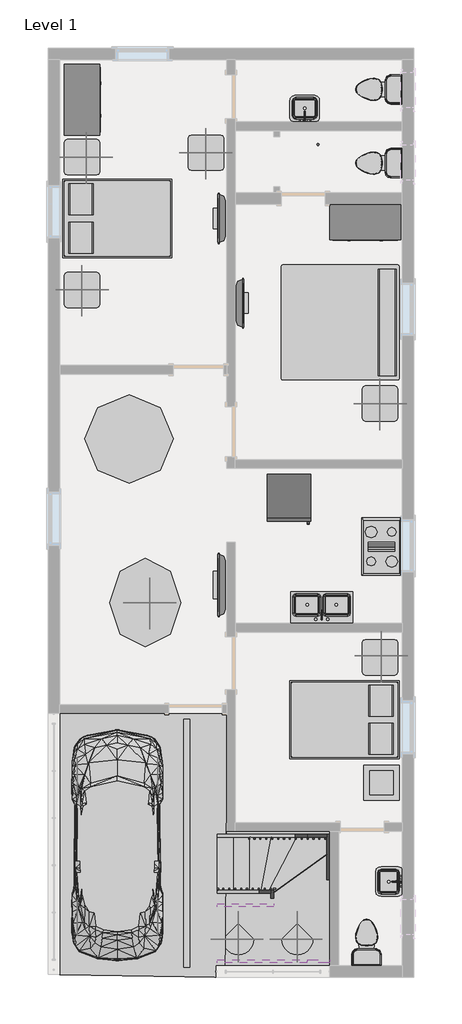
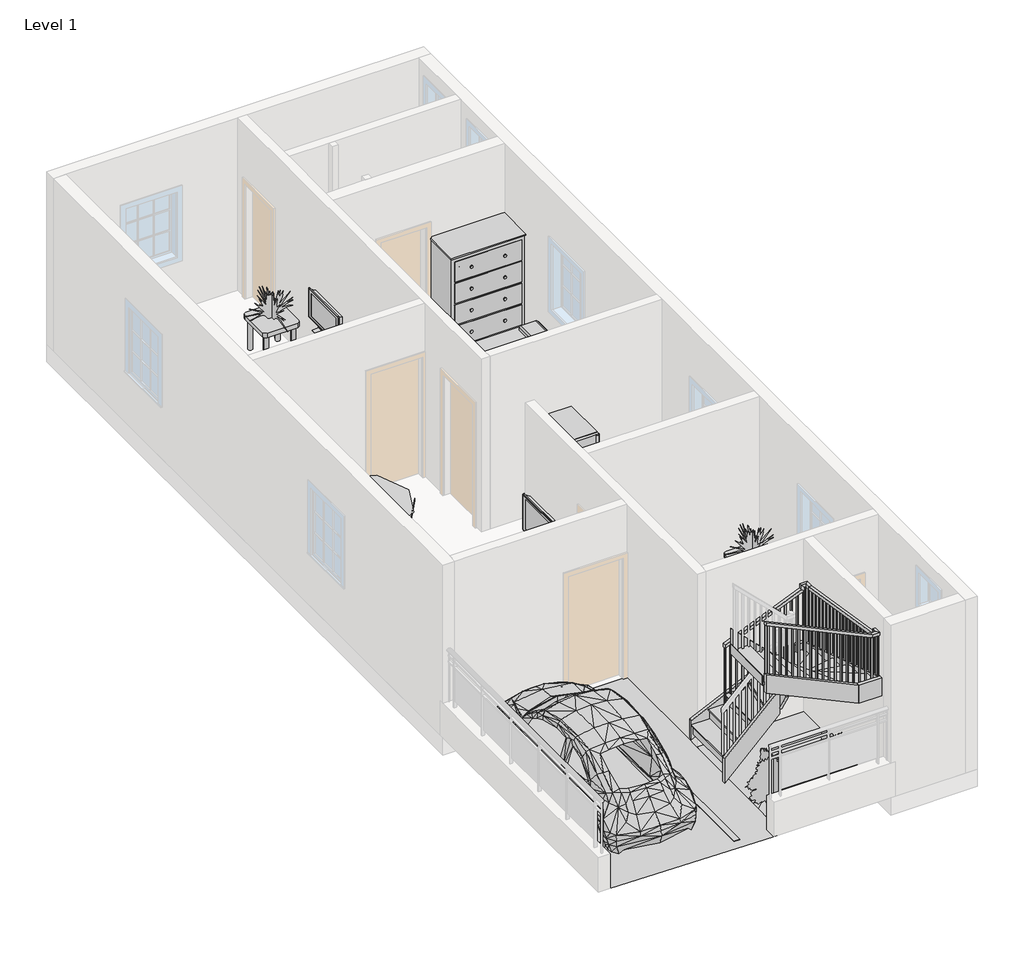
# One storey, part 3 of 3: 16 furniture elements, 10 flow terminals, 8 geographic elements, 8 members, 6 proxies, 1 railing, 1 stair flight.
"""IFC4 building model written with IfcOpenShell, lengths in millimetres."""

from ifc_helpers import new_model, si_unit, frame, origin, place, context, project, spatial, polyline, outline, extrude, faceted_brep, triangles, transform, mapped, element, save
from components import proxy_bb1e6e30, parking_space_9_x_18_90_deg_fdd9e8f5, rpc_beetle_rpc_beetle_3ce7ba48, proxy_a13a33b2, flow_terminal_2b63360b, flow_terminal_accce45a, flow_terminal_a53be723, flow_terminal_d49f872f, flow_terminal_62a433f7, toilet_domestic_3d_toilet_domestic_3d_f7549cf7, toilet_domestic_3d_toilet_domestic_3d_183bbd19, furniture_c8abb964, furniture_1fc5af50, furniture_9fa109b2, furniture_56245f3a, furniture_7a3aaa4f, furniture_b5c51a22, furniture_bbcc68ce, furniture_743965d2, furniture_31d08a24, rpc_plant_tropical_agave_1_5_93a2a214, rpc_plant_tropical_jungle_flame_3_9c4808c2, stair_flight_89efee2b

model = new_model("IFC4")

# Units and contexts
model_context = context("Model", 3, world=origin())
ifc_project = project(units=[si_unit("LENGTHUNIT", "METRE", prefix="MILLI")], contexts=[model_context])

# Site, building, storey
site = spatial("IfcSite", under=ifc_project)
building = spatial("IfcBuilding", under=site)
storey = spatial("IfcBuildingStorey", under=building, Name="Level 1", Elevation=0.0)

# Proxies
placement = place(None, origin())
element("IfcBuildingElementProxy", 1, Name="Building Element Proxy", at=placement, inside=storey, context=model_context, shape_type="Tessellation", body=[
    triangles([(-14717.9109375, 1512.0104702, 0.0), (-11644.5113251, 1512.0104702, 0.0), (-11665.5135315, -2272.5896267, 0.0), (-14514.7117126, -2272.5896267, 0.0), (-14514.7117126, -2983.7896751, 0.0), (-11822.3109375, -3034.5894814, 0.0), (-11675.0896912, -3034.5894814, 0.0)], [[1, 5, 4], [4, 5, 6], [1, 4, 2], [6, 7, 3], [2, 4, 3], [3, 4, 6]], closed=False),
])
element("IfcBuildingElementProxy", 2, Name="Building Element Proxy", at=placement, inside=storey, context=model_context, shape_type="Tessellation", body=[
    triangles([(-11644.5113251, -519.9895904, 0.0), (-9968.1113251, -519.9895904, 0.0), (-9968.1113251, -2272.5896267, 0.0), (-11568.3113251, -2272.5896267, 0.0), (-11664.9972839, -2272.5896267, 0.0), (-11667.5389893, -855.5340437, 0.0), (-9866.5117126, -2475.7895782, 0.0), (-9866.5117126, -519.9895904, 0.0), (-11653.0654541, -2831.3896751, 0.0), (-11670.8166962, -2831.3896751, 0.0), (-9866.5117126, -2831.3896751, 0.0)], [[10, 9, 5], [3, 9, 11], [1, 6, 2], [5, 6, 10], [5, 4, 6], [5, 9, 4], [3, 11, 7], [3, 4, 9], [3, 6, 4], [3, 7, 8], [2, 6, 3], [2, 3, 8]], closed=False),
])
proxy_shape = proxy_bb1e6e30(model_context)
element("IfcBuildingElementProxy", 3, Name="Cook Top-4 Unit : 36\" x 20\"", ObjectType="Cook Top-4 Unit : 36\" x 20\"", at=placement, inside=storey, context=model_context, shape_type="MappedRepresentation", body=[
    mapped(proxy_shape, transform((-8977.5112155, 4382.2104001, 0.0), x_axis=(0.0, -1.0000000000000004, 0.0), y_axis=(1.0000000000000004, 0.0, 0.0), z_axis=(0.0, 0.0, 1.0))),
])
parking_space_9_x_18_90_deg_shape = parking_space_9_x_18_90_deg_fdd9e8f5(model_context)
element("IfcBuildingElementProxy", 4, Name="Parking Space : 9' x 18' - 90 deg", ObjectType="Parking Space : 9' x 18' - 90 deg", at=placement, inside=storey, context=model_context, shape_type="MappedRepresentation", body=[
    mapped(parking_space_9_x_18_90_deg_shape, transform((-12330.3112155, -2856.7895999, 0.0), x_axis=(-1.0000000000000002, 0.0, 0.0), y_axis=(0.0, -1.0000000000000002, 0.0), z_axis=(0.0, 0.0, 1.0))),
])
rpc_beetle_rpc_beetle_shape = rpc_beetle_rpc_beetle_3ce7ba48(model_context)
element("IfcBuildingElementProxy", 5, Name="RPC Beetle : RPC Beetle", ObjectType="RPC Beetle : RPC Beetle", at=placement, inside=storey, context=model_context, shape_type="MappedRepresentation", body=[
    mapped(rpc_beetle_rpc_beetle_shape, transform((-13524.1112155, -1993.1895999, 0.0), x_axis=(1.0, 0.0, 0.0), y_axis=(0.0, 1.0, 0.0), z_axis=(0.0, 0.0, 1.0))),
])
proxy_2_shape = proxy_a13a33b2(model_context)
element("IfcBuildingElementProxy", 6, Name="Refrigerator : 30\" x 32\" RH", ObjectType="Refrigerator : 30\" x 32\" RH", at=placement, inside=storey, context=model_context, shape_type="MappedRepresentation", body=[
    mapped(proxy_2_shape, transform((-10569.7737155, 5238.2614286, 0.0), x_axis=(1.0, 0.0, 0.0), y_axis=(0.0, 1.0, 0.0), z_axis=(0.0, 0.0, 1.0))),
])

# Flow terminals
flow_terminal_shape = flow_terminal_2b63360b(model_context)
element("IfcFlowTerminal", 7, ObjectType="Floor Drain - Rectangular : 5\"x5\" Strainer - 2\" Drain", at=placement, inside=storey, context=model_context, shape_type="MappedRepresentation", body=[
    mapped(flow_terminal_shape, transform((-9587.1112155, 12586.4104001, 0.0), x_axis=(1.0, 0.0, 0.0), y_axis=(0.0, 1.0, 0.0), z_axis=(0.0, 0.0, 1.0))),
])
element("IfcFlowTerminal", 8, ObjectType="Floor Drain - Rectangular : 5\"x5\" Strainer - 2\" Drain", at=placement, inside=storey, context=model_context, shape_type="MappedRepresentation", body=[
    mapped(flow_terminal_shape, transform((-9510.9112155, 11367.2104001, 0.0), x_axis=(1.0, 0.0, 0.0), y_axis=(0.0, 1.0, 0.0), z_axis=(0.0, 0.0, 1.0))),
])
flow_terminal_2_shape = flow_terminal_accce45a(model_context)
element("IfcFlowTerminal", 9, ObjectType="Floor Drain - Round : 5\" Strainer - 2\" Drain", at=placement, inside=storey, context=model_context, shape_type="MappedRepresentation", body=[
    mapped(flow_terminal_2_shape, transform((-8799.7112155, -2145.5895999, 0.0), x_axis=(1.0, 0.0, 0.0), y_axis=(0.0, 1.0, 0.0), z_axis=(0.0, 0.0, 1.0))),
])
flow_terminal_3_shape = flow_terminal_a53be723(model_context)
element("IfcFlowTerminal", 10, ObjectType="Sink Kitchen-Double : 42\" x 21\"", at=placement, inside=storey, context=model_context, shape_type="MappedRepresentation", body=[
    mapped(flow_terminal_3_shape, transform((-9990.521975, 3343.1558012, 0.0), x_axis=(-1.0000000000000004, 0.0, 0.0), y_axis=(0.0, -1.0000000000000004, 0.0), z_axis=(0.0, 0.0, 1.0))),
])
flow_terminal_4_shape = flow_terminal_d49f872f(model_context)
element("IfcFlowTerminal", 11, ObjectType="Sink Vanity-Round : 19\" x 19\"", at=placement, inside=storey, context=model_context, shape_type="MappedRepresentation", body=[
    mapped(flow_terminal_4_shape, transform((-10166.3629561, 11222.9262428, 609.6), x_axis=(1.0000000000000004, 0.0, 0.0), y_axis=(0.0, 1.0000000000000004, 0.0), z_axis=(0.0, 0.0, 1.0))),
])
flow_terminal_5_shape = flow_terminal_62a433f7(model_context)
element("IfcFlowTerminal", 12, ObjectType="Sink Vanity-Square : 20\" x 18\"", at=placement, inside=storey, context=model_context, shape_type="MappedRepresentation", body=[
    mapped(flow_terminal_5_shape, transform((-10282.621975, 11877.5558012, 0.0), x_axis=(-1.0000000000000004, 0.0, 0.0), y_axis=(0.0, -1.0000000000000004, 0.0), z_axis=(0.0, 0.0, 1.0))),
])
element("IfcFlowTerminal", 13, ObjectType="Sink Vanity-Square : 20\" x 18\"", at=placement, inside=storey, context=model_context, shape_type="MappedRepresentation", body=[
    mapped(flow_terminal_5_shape, transform((-8802.0566166, -1367.9003593, 0.0), x_axis=(0.0, -1.0000000000000004, 0.0), y_axis=(1.0000000000000004, 0.0, 0.0), z_axis=(0.0, 0.0, 1.0))),
])
toilet_domestic_3d_toilet_domestic_3d_shape = toilet_domestic_3d_toilet_domestic_3d_f7549cf7(model_context)
toilet_domestic_3d_toilet_domestic_3d_2_shape = toilet_domestic_3d_toilet_domestic_3d_183bbd19(model_context)
element("IfcFlowTerminal", 14, ObjectType="Toilet-Domestic-3D : Toilet-Domestic-3D", at=placement, inside=storey, context=model_context, shape_type="MappedRepresentation", body=[
    mapped(toilet_domestic_3d_toilet_domestic_3d_shape, transform((-9116.6072429, 12256.2104001, 0.0), x_axis=(0.0, -1.0000000000000004, 0.0), y_axis=(1.0000000000000004, 0.0, 0.0), z_axis=(0.0, 0.0, 1.0))),
    mapped(toilet_domestic_3d_toilet_domestic_3d_2_shape, transform((-9116.6072429, 12256.2104001, 0.0), x_axis=(0.0, -1.0000000000000004, 0.0), y_axis=(1.0000000000000004, 0.0, 0.0), z_axis=(0.0, 0.0, 1.0))),
])
element("IfcFlowTerminal", 15, ObjectType="Toilet-Domestic-3D : Toilet-Domestic-3D", at=placement, inside=storey, context=model_context, shape_type="MappedRepresentation", body=[
    mapped(toilet_domestic_3d_toilet_domestic_3d_shape, transform((-9116.6072429, 10986.2104001, 0.0), x_axis=(0.0, -1.0000000000000004, 0.0), y_axis=(1.0000000000000004, 0.0, 0.0), z_axis=(0.0, 0.0, 1.0))),
    mapped(toilet_domestic_3d_toilet_domestic_3d_2_shape, transform((-9116.6072429, 10986.2104001, 0.0), x_axis=(0.0, -1.0000000000000004, 0.0), y_axis=(1.0000000000000004, 0.0, 0.0), z_axis=(0.0, 0.0, 1.0))),
])
element("IfcFlowTerminal", 16, ObjectType="Toilet-Domestic-3D : Toilet-Domestic-3D", at=placement, inside=storey, context=model_context, shape_type="MappedRepresentation", body=[
    mapped(toilet_domestic_3d_toilet_domestic_3d_shape, transform((-9231.5112155, -2336.6935725, 0.0), x_axis=(-1.0000000000000002, 0.0, 0.0), y_axis=(0.0, -1.0000000000000002, 0.0), z_axis=(0.0, 0.0, 1.0))),
    mapped(toilet_domestic_3d_toilet_domestic_3d_2_shape, transform((-9231.5112155, -2336.6935725, 0.0), x_axis=(-1.0000000000000002, 0.0, 0.0), y_axis=(0.0, -1.0000000000000002, 0.0), z_axis=(0.0, 0.0, 1.0))),
])

# Furniture
furniture_shape = furniture_c8abb964(model_context)
element("IfcFurniture", 17, ObjectType="Bed-Box : Double 53\" x 74\"", at=placement, inside=storey, context=model_context, shape_type="MappedRepresentation", body=[
    mapped(furniture_shape, transform((-13758.5407237, 9694.5579411, 0.0), x_axis=(0.0, 1.0000000000000002, 0.0), y_axis=(-1.0000000000000002, 0.0, 0.0), z_axis=(0.0, 0.0, 1.0))),
])
element("IfcFurniture", 18, ObjectType="Bed-Box : Double 53\" x 74\"", at=placement, inside=storey, context=model_context, shape_type="MappedRepresentation", body=[
    mapped(furniture_shape, transform((-9378.0817073, 1740.6104001, 0.0), x_axis=(0.0, -1.0000000000000002, 0.0), y_axis=(1.0000000000000002, 0.0, 0.0), z_axis=(0.0, 0.0, 1.0))),
])
furniture_2_shape = furniture_1fc5af50(model_context)
element("IfcFurniture", 19, ObjectType="Bed-Standard.0001 : King 78\" x 80\"", at=placement, inside=storey, context=model_context, shape_type="MappedRepresentation", body=[
    mapped(furniture_2_shape, transform((-9643.1161336, 8514.4989247, 0.0), x_axis=(0.0, -1.0, 0.0), y_axis=(1.0, 0.0, 0.0), z_axis=(0.0, 0.0, 1.0))),
])
furniture_3_shape = furniture_9fa109b2(model_context)
element("IfcFurniture", 20, ObjectType="Dresser : 48\" x 72\" x 24\"", at=placement, inside=storey, context=model_context, shape_type="MappedRepresentation", body=[
    mapped(furniture_3_shape, transform((-14496.8741696, 12347.6036599, 0.0), x_axis=(0.0, 1.0000000000000002, 0.0), y_axis=(-1.0000000000000002, 0.0, 0.0), z_axis=(0.0, 0.0, 1.0))),
])
element("IfcFurniture", 21, ObjectType="Dresser : 48\" x 72\" x 24\"", at=placement, inside=storey, context=model_context, shape_type="MappedRepresentation", body=[
    mapped(furniture_3_shape, transform((-8987.7179557, 10333.3733542, 0.0), x_axis=(1.0, 0.0, 0.0), y_axis=(0.0, 1.0, 0.0), z_axis=(0.0, 0.0, 1.0))),
])
furniture_4_shape = furniture_56245f3a(model_context)
element("IfcFurniture", 22, ObjectType="TV - Flat Screen : 32\"", at=placement, inside=storey, context=model_context, shape_type="MappedRepresentation", body=[
    mapped(furniture_4_shape, transform((-11722.0998392, 10029.765886, 914.4), x_axis=(0.0, -1.0000000000000002, 0.0), y_axis=(1.0000000000000002, 0.0, 0.0), z_axis=(0.0, 0.0, 1.0))),
])
element("IfcFurniture", 23, ObjectType="TV - Flat Screen : 32\"", at=placement, inside=storey, context=model_context, shape_type="MappedRepresentation", body=[
    mapped(furniture_4_shape, transform((-11420.9593185, 8577.1549142, 914.4), x_axis=(0.0, 1.0000000000000002, 0.0), y_axis=(-1.0000000000000002, 0.0, 0.0), z_axis=(0.0, 0.0, 1.0))),
])
furniture_5_shape = furniture_7a3aaa4f(model_context)
element("IfcFurniture", 24, ObjectType="TV - Flat Screen : 42\"", at=placement, inside=storey, context=model_context, shape_type="MappedRepresentation", body=[
    mapped(furniture_5_shape, transform((-11722.0998392, 3717.865886, 914.4), x_axis=(0.0, -1.0000000000000004, 0.0), y_axis=(1.0000000000000004, 0.0, 0.0), z_axis=(0.0, 0.0, 1.0))),
])
furniture_6_shape = furniture_b5c51a22(model_context)
element("IfcFurniture", 25, ObjectType="Table-Coffee : 24\" x 24\" x 24\"", at=placement, inside=storey, context=model_context, shape_type="MappedRepresentation", body=[
    mapped(furniture_6_shape, transform((-8995.7769822, 222.9993223, 0.0), x_axis=(1.0, 0.0, 0.0), y_axis=(0.0, 1.0, 0.0), z_axis=(0.0, 0.0, 1.0))),
])
furniture_7_shape = furniture_bbcc68ce(model_context)
element("IfcFurniture", 26, ObjectType="Table-Dining Round w Chairs : 60\" Diameter", at=placement, inside=storey, context=model_context, shape_type="MappedRepresentation", body=[
    mapped(furniture_7_shape, transform((-13424.5931827, 6421.2890886, 0.0), x_axis=(1.0, 0.0, 0.0), y_axis=(0.0, 1.0, 0.0), z_axis=(0.0, 0.0, 1.0))),
])
furniture_8_shape = furniture_743965d2(model_context)
element("IfcFurniture", 27, ObjectType="Table-Ellipse : 60\" x 48\"", at=placement, inside=storey, context=model_context, shape_type="MappedRepresentation", body=[
    mapped(furniture_8_shape, transform((-13041.5112155, 3417.0104001, 0.0), x_axis=(0.0, 1.0000000000000002, 0.0), y_axis=(-1.0000000000000002, 0.0, 0.0), z_axis=(0.0, 0.0, 1.0))),
])
furniture_9_shape = furniture_31d08a24(model_context)
element("IfcFurniture", 28, ObjectType="Table-End : 24\" x 24\"", at=placement, inside=storey, context=model_context, shape_type="MappedRepresentation", body=[
    mapped(furniture_9_shape, transform((-14442.2448458, 10935.4104001, 0.0), x_axis=(1.0, 0.0, 0.0), y_axis=(0.0, 1.0, 0.0), z_axis=(0.0, 0.0, 1.0))),
])
element("IfcFurniture", 29, ObjectType="Table-End : 24\" x 24\"", at=placement, inside=storey, context=model_context, shape_type="MappedRepresentation", body=[
    mapped(furniture_9_shape, transform((-14442.2448458, 8649.4104001, 0.0), x_axis=(1.0, 0.0, 0.0), y_axis=(0.0, 1.0, 0.0), z_axis=(0.0, 0.0, 1.0))),
])
element("IfcFurniture", 30, ObjectType="Table-End : 24\" x 24\"", at=placement, inside=storey, context=model_context, shape_type="MappedRepresentation", body=[
    mapped(furniture_9_shape, transform((-12308.6448458, 11011.6104001, 0.0), x_axis=(1.0, 0.0, 0.0), y_axis=(0.0, 1.0, 0.0), z_axis=(0.0, 0.0, 1.0))),
])
element("IfcFurniture", 31, ObjectType="Table-End : 24\" x 24\"", at=placement, inside=storey, context=model_context, shape_type="MappedRepresentation", body=[
    mapped(furniture_9_shape, transform((-9311.4448458, 6693.6104001, 0.0), x_axis=(1.0, 0.0, 0.0), y_axis=(0.0, 1.0, 0.0), z_axis=(0.0, 0.0, 1.0))),
])
element("IfcFurniture", 32, ObjectType="Table-End : 24\" x 24\"", at=placement, inside=storey, context=model_context, shape_type="MappedRepresentation", body=[
    mapped(furniture_9_shape, transform((-9311.4448458, 2324.8104001, 0.0), x_axis=(1.0, 0.0, 0.0), y_axis=(0.0, 1.0, 0.0), z_axis=(0.0, 0.0, 1.0))),
])

# Geographic elements
rpc_plant_tropical_agave_1_5_shape = rpc_plant_tropical_agave_1_5_93a2a214(model_context)
element("IfcGeographicElement", 33, ObjectType="RPC Plant - Tropical : Agave - 1.5'", at=placement, inside=storey, context=model_context, shape_type="MappedRepresentation", body=[
    mapped(rpc_plant_tropical_agave_1_5_shape, transform((-14057.5112155, 11087.8104001, 609.6), x_axis=(1.0, 0.0, 0.0), y_axis=(0.0, 1.0, 0.0), z_axis=(0.0, 0.0, 1.0))),
])
element("IfcGeographicElement", 34, ObjectType="RPC Plant - Tropical : Agave - 1.5'", at=placement, inside=storey, context=model_context, shape_type="MappedRepresentation", body=[
    mapped(rpc_plant_tropical_agave_1_5_shape, transform((-14133.7112155, 8801.8104001, 609.6), x_axis=(1.0, 0.0, 0.0), y_axis=(0.0, 1.0, 0.0), z_axis=(0.0, 0.0, 1.0))),
])
element("IfcGeographicElement", 35, ObjectType="RPC Plant - Tropical : Agave - 1.5'", at=placement, inside=storey, context=model_context, shape_type="MappedRepresentation", body=[
    mapped(rpc_plant_tropical_agave_1_5_shape, transform((-12000.1112155, 11164.0104001, 609.6), x_axis=(1.0, 0.0, 0.0), y_axis=(0.0, 1.0, 0.0), z_axis=(0.0, 0.0, 1.0))),
])
element("IfcGeographicElement", 36, ObjectType="RPC Plant - Tropical : Agave - 1.5'", at=placement, inside=storey, context=model_context, shape_type="MappedRepresentation", body=[
    mapped(rpc_plant_tropical_agave_1_5_shape, transform((-9002.9112155, 6846.0104001, 609.6), x_axis=(1.0, 0.0, 0.0), y_axis=(0.0, 1.0, 0.0), z_axis=(0.0, 0.0, 1.0))),
])
element("IfcGeographicElement", 37, ObjectType="RPC Plant - Tropical : Agave - 1.5'", at=placement, inside=storey, context=model_context, shape_type="MappedRepresentation", body=[
    mapped(rpc_plant_tropical_agave_1_5_shape, transform((-12965.3112155, 3417.0104001, 762.0), x_axis=(1.0, 0.0, 0.0), y_axis=(0.0, 1.0, 0.0), z_axis=(0.0, 0.0, 1.0))),
])
element("IfcGeographicElement", 38, ObjectType="RPC Plant - Tropical : Agave - 1.5'", at=placement, inside=storey, context=model_context, shape_type="MappedRepresentation", body=[
    mapped(rpc_plant_tropical_agave_1_5_shape, transform((-8977.5112155, 2502.6104001, 609.6), x_axis=(1.0, 0.0, 0.0), y_axis=(0.0, 1.0, 0.0), z_axis=(0.0, 0.0, 1.0))),
])
rpc_plant_tropical_jungle_flame_3_shape = rpc_plant_tropical_jungle_flame_3_9c4808c2(model_context)
element("IfcGeographicElement", 39, ObjectType="RPC Plant - Tropical : Jungle Flame - 3'", at=placement, inside=storey, context=model_context, shape_type="MappedRepresentation", body=[
    mapped(rpc_plant_tropical_jungle_flame_3_shape, transform((-11441.3112155, -2374.1895999, 0.0), x_axis=(1.0, 0.0, 0.0), y_axis=(0.0, 1.0, 0.0), z_axis=(0.0, 0.0, 1.0))),
])
element("IfcGeographicElement", 40, ObjectType="RPC Plant - Tropical : Jungle Flame - 3'", at=placement, inside=storey, context=model_context, shape_type="MappedRepresentation", body=[
    mapped(rpc_plant_tropical_jungle_flame_3_shape, transform((-10425.3112155, -2374.1895999, 0.0), x_axis=(1.0, 0.0, 0.0), y_axis=(0.0, 1.0, 0.0), z_axis=(0.0, 0.0, 1.0))),
])

# Members
element("IfcMember", 41, ObjectType="Stringer - 2\" Width", at=placement, inside=storey, context=model_context, shape_type="SweptSolid", body=[
    extrude(outline(polyline([(577.8751786, -11800.6429074), (241.2701641, -11800.6429074), (965.2955504, -10255.5493466), (1301.9005649, -10255.5493466), (577.8751786, -11800.6429074)])), frame((0.0, -621.5895999, 0.0), z_axis=(0.0, 1.0, 0.0), x_axis=(0.0, 0.0, 1.0)), (0.0, 0.0, 1.0), 50.8),
])
element("IfcMember", 42, ObjectType="Stringer - 2\" Width", at=placement, inside=storey, context=model_context, shape_type="SweptSolid", body=[
    extrude(outline(polyline([(-10255.5493466, -621.5895999), (-10255.5493466, -570.7895999), (-9917.3112155, -570.7895999), (-9917.3112155, -621.5895999), (-10255.5493466, -621.5895999)])), frame((0.0, 0.0, 965.2955504), z_axis=(0.0, 0.0, 1.0), x_axis=(1.0, 0.0, 0.0)), (0.0, 0.0, 1.0), 336.6050145),
])
element("IfcMember", 43, ObjectType="Stringer - 2\" Width", at=placement, inside=storey, context=model_context, shape_type="SweptSolid", body=[
    extrude(outline(polyline([(-570.7895999, 1285.6001408), (-570.7895999, 997.1005649), (-720.7093972, 997.1005649), (-2729.7895999, 1641.7631511), (-2729.7895999, 1969.9972697), (-2703.7018424, 1969.9972697), (-570.7895999, 1285.6001408)])), frame((-9917.3112155, 0.0, 0.0), z_axis=(1.0, 0.0, 0.0), x_axis=(0.0, 1.0, 0.0)), (0.0, 0.0, 1.0), 50.8),
])
element("IfcMember", 44, ObjectType="Stringer - 2\" Width", at=placement, inside=storey, context=model_context, shape_type="SweptSolid", body=[
    extrude(outline(polyline([(-9866.5112155, -2729.7895999), (-9866.5112155, -2780.5895999), (-10255.5493466, -2780.5895999), (-10255.5493466, -2729.7895999), (-9866.5112155, -2729.7895999)])), frame((0.0, 0.0, 1649.8904473), z_axis=(0.0, 0.0, 1.0), x_axis=(1.0, 0.0, 0.0)), (0.0, 0.0, 1.0), 320.1068224),
])
element("IfcMember", 45, ObjectType="Stringer - 2\" Width", at=placement, inside=storey, context=model_context, shape_type="SweptSolid", body=[
    extrude(outline(polyline([(1649.8904473, -10255.5493466), (1969.9972697, -10255.5493466), (2694.022656, -11800.6429074), (2373.9158336, -11800.6429074), (1649.8904473, -10255.5493466)])), frame((0.0, -2780.5895999, 0.0), z_axis=(0.0, 1.0, 0.0), x_axis=(0.0, 0.0, 1.0)), (0.0, 0.0, 1.0), 50.8),
])
element("IfcMember", 46, ObjectType="Stringer - 2\" Width", at=placement, inside=storey, context=model_context, shape_type="SweptSolid", body=[
    extrude(outline(polyline([(489.3391875, -11800.6429074), (61.3897561, -11800.6429074), (966.2551233, -10882.5112155), (1394.2045547, -10882.5112155), (489.3391875, -11800.6429074)])), frame((0.0, -1586.7895999, 0.0), z_axis=(0.0, 1.0, 0.0), x_axis=(0.0, 0.0, 1.0)), (0.0, 0.0, 1.0), 50.8),
])
element("IfcMember", 47, ObjectType="Stringer - 2\" Width", at=placement, inside=storey, context=model_context, shape_type="SweptSolid", body=[
    extrude(outline(polyline([(-1535.9895999, 1573.2682978), (-1535.9895999, 1016.3211008), (-1563.063862, 1016.3211008), (-1764.5895999, 1360.465107), (-1764.5895999, 1947.8002622), (-1755.3100853, 1947.8002622), (-1535.9895999, 1573.2682978)])), frame((-10882.5112155, 0.0, 0.0), z_axis=(1.0, 0.0, 0.0), x_axis=(0.0, 1.0, 0.0)), (0.0, 0.0, 1.0), 50.8),
])
element("IfcMember", 48, ObjectType="Stringer - 2\" Width", at=placement, inside=storey, context=model_context, shape_type="SweptSolid", body=[
    extrude(outline(polyline([(1519.8508308, -10831.7112155), (1947.8002622, -10831.7112155), (2902.731607, -11800.6429074), (2474.7821756, -11800.6429074), (1519.8508308, -10831.7112155)])), frame((0.0, -1815.3895999, 0.0), z_axis=(0.0, 1.0, 0.0), x_axis=(0.0, 0.0, 1.0)), (0.0, 0.0, 1.0), 50.8),
])

# Railing
element("IfcRailing", 49, ObjectType="Handrail - Rectangular", at=placement, inside=storey, context=model_context, shape_type="SolidModel", body=[
    faceted_brep([(-11264.9343115, -621.5895999, 1751.3482604), (-11264.9343115, -621.5895999, 1696.2325103), (-11264.9343115, -672.3895999, 1696.2325103), (-11264.9343115, -672.3895999, 1751.3482604), (-9993.5112155, -621.5895999, 2286.4480794), (-9942.7112155, -621.5895999, 2252.7123647), (-9942.7112155, -672.3895999, 2252.7123647), (-9993.5112155, -672.3895999, 2286.4480794), (-9866.5112155, -752.6490579, 2309.5259032), (-9866.5112155, -748.5895999, 2360.3259032), (-9866.5112155, -2602.7895999, 2658.5708374), (-9866.5112155, -2653.5895999, 2615.2889745), (-9917.3112155, -752.6490579, 2309.5259032), (-9917.3112155, -2653.5895999, 2615.2889745), (-9917.3112155, -748.5895999, 2360.3259032), (-9917.3112155, -2602.7895999, 2658.5708374), (-11771.5112155, -2729.7895999, 3571.6748454), (-11771.5112155, -2678.9895999, 3571.6748454), (-11771.5112155, -2678.9895999, 3515.5740097), (-11771.5112155, -2729.7895999, 3515.5740097), (-10004.8233702, -2729.7895999, 2687.7103241), (-9993.5112155, -2729.7895999, 2738.5103241), (-10004.8233702, -2678.9895999, 2687.7103241), (-9993.5112155, -2678.9895999, 2738.5103241), (-9993.5112155, -621.5895999, 2360.3259032), (-9942.7112155, -621.5895999, 2309.5259032), (-9942.7112155, -672.3895999, 2309.5259032), (-9993.5112155, -672.3895999, 2360.3259032), (-9866.5112155, -621.5895999, 2360.3259032), (-9866.5112155, -621.5895999, 2309.5259032), (-9917.3112155, -672.3895999, 2309.5259032), (-9917.3112155, -672.3895999, 2360.3259032), (-9866.5112155, -2602.7895999, 2738.5103241), (-9866.5112155, -2653.5895999, 2687.7103241), (-9917.3112155, -2653.5895999, 2687.7103241), (-9917.3112155, -2602.7895999, 2738.5103241), (-9866.5112155, -2729.7895999, 2738.5103241), (-9866.5112155, -2729.7895999, 2687.7103241), (-9917.3112155, -2678.9895999, 2687.7103241), (-9917.3112155, -2678.9895999, 2738.5103241)], [[[0, 1, 2, 3]], [[1, 0, 4, 5]], [[2, 1, 5, 6]], [[3, 2, 6, 7]], [[0, 3, 7, 4]], [[8, 9, 10, 11]], [[12, 8, 11, 13]], [[14, 12, 13, 15]], [[9, 14, 15, 10]], [[16, 17, 18, 19]], [[20, 21, 16, 19]], [[22, 20, 19, 18]], [[23, 22, 18, 17]], [[21, 23, 17, 16]], [[5, 4, 24, 25]], [[6, 5, 25, 26]], [[7, 6, 26, 27]], [[4, 7, 27, 24]], [[25, 24, 28, 29]], [[26, 25, 29, 30]], [[27, 26, 30, 31]], [[24, 27, 31, 28]], [[29, 28, 9, 8]], [[30, 29, 8, 12]], [[31, 30, 12, 14]], [[28, 31, 14, 9]], [[11, 10, 32, 33]], [[13, 11, 33, 34]], [[15, 13, 34, 35]], [[10, 15, 35, 32]], [[33, 32, 36, 37]], [[34, 33, 37, 38]], [[35, 34, 38, 39]], [[32, 35, 39, 36]], [[37, 36, 21, 20]], [[38, 37, 20, 22]], [[39, 38, 22, 23]], [[36, 39, 23, 21]]]),
    extrude(outline(polyline([(3496.2326904, -11730.2362155), (2540.0, -11730.2362155), (2540.0, -11711.1862155), (3487.3059277, -11711.1862155), (3496.2326904, -11730.2362155)])), frame((0.0, -2713.9145999, 0.0), z_axis=(0.0, 1.0, 0.0), x_axis=(0.0, 0.0, 1.0)), (0.0, 0.0, 1.0), 19.05),
    extrude(outline(polyline([(3448.6232892, -11628.6362155), (2540.0, -11628.6362155), (2540.0, -11609.5862155), (3439.6965265, -11609.5862155), (3448.6232892, -11628.6362155)])), frame((0.0, -2713.9145999, 0.0), z_axis=(0.0, 1.0, 0.0), x_axis=(0.0, 0.0, 1.0)), (0.0, 0.0, 1.0), 19.05),
    extrude(outline(polyline([(3401.013888, -11527.0362155), (2370.6666667, -11527.0362155), (2370.6666667, -11507.9862155), (3392.0871253, -11507.9862155), (3401.013888, -11527.0362155)])), frame((0.0, -2713.9145999, 0.0), z_axis=(0.0, 1.0, 0.0), x_axis=(0.0, 0.0, 1.0)), (0.0, 0.0, 1.0), 19.05),
    extrude(outline(polyline([(3353.4044868, -11425.4362155), (2370.6666667, -11425.4362155), (2370.6666667, -11406.3862155), (3344.477724, -11406.3862155), (3353.4044868, -11425.4362155)])), frame((0.0, -2713.9145999, 0.0), z_axis=(0.0, 1.0, 0.0), x_axis=(0.0, 0.0, 1.0)), (0.0, 0.0, 1.0), 19.05),
    extrude(outline(polyline([(3305.7950856, -11323.8362155), (2370.6666667, -11323.8362155), (2370.6666667, -11304.7862155), (3296.8683228, -11304.7862155), (3305.7950856, -11323.8362155)])), frame((0.0, -2713.9145999, 0.0), z_axis=(0.0, 1.0, 0.0), x_axis=(0.0, 0.0, 1.0)), (0.0, 0.0, 1.0), 19.05),
    extrude(outline(polyline([(3258.1856843, -11222.2362155), (2201.3333333, -11222.2362155), (2201.3333333, -11203.1862155), (3249.2589216, -11203.1862155), (3258.1856843, -11222.2362155)])), frame((0.0, -2713.9145999, 0.0), z_axis=(0.0, 1.0, 0.0), x_axis=(0.0, 0.0, 1.0)), (0.0, 0.0, 1.0), 19.05),
    extrude(outline(polyline([(3210.5762831, -11120.6362155), (2201.3333333, -11120.6362155), (2201.3333333, -11101.5862155), (3201.6495204, -11101.5862155), (3210.5762831, -11120.6362155)])), frame((0.0, -2713.9145999, 0.0), z_axis=(0.0, 1.0, 0.0), x_axis=(0.0, 0.0, 1.0)), (0.0, 0.0, 1.0), 19.05),
    extrude(outline(polyline([(3162.9668819, -11019.0362155), (2201.3333333, -11019.0362155), (2201.3333333, -10999.9862155), (3154.0401192, -10999.9862155), (3162.9668819, -11019.0362155)])), frame((0.0, -2713.9145999, 0.0), z_axis=(0.0, 1.0, 0.0), x_axis=(0.0, 0.0, 1.0)), (0.0, 0.0, 1.0), 19.05),
    extrude(outline(polyline([(3115.3574807, -10917.4362155), (2201.3333333, -10917.4362155), (2201.3333333, -10898.3862155), (3106.430718, -10898.3862155), (3115.3574807, -10917.4362155)])), frame((0.0, -2713.9145999, 0.0), z_axis=(0.0, 1.0, 0.0), x_axis=(0.0, 0.0, 1.0)), (0.0, 0.0, 1.0), 19.05),
    extrude(outline(polyline([(3067.7480795, -10815.8362155), (2032.0, -10815.8362155), (2032.0, -10796.7862155), (3058.8213168, -10796.7862155), (3067.7480795, -10815.8362155)])), frame((0.0, -2713.9145999, 0.0), z_axis=(0.0, 1.0, 0.0), x_axis=(0.0, 0.0, 1.0)), (0.0, 0.0, 1.0), 19.05),
    extrude(outline(polyline([(3020.1386783, -10714.2362155), (2032.0, -10714.2362155), (2032.0, -10695.1862155), (3011.2119155, -10695.1862155), (3020.1386783, -10714.2362155)])), frame((0.0, -2713.9145999, 0.0), z_axis=(0.0, 1.0, 0.0), x_axis=(0.0, 0.0, 1.0)), (0.0, 0.0, 1.0), 19.05),
    extrude(outline(polyline([(2972.5292771, -10612.6362155), (2032.0, -10612.6362155), (2032.0, -10593.5862155), (2963.6025143, -10593.5862155), (2972.5292771, -10612.6362155)])), frame((0.0, -2713.9145999, 0.0), z_axis=(0.0, 1.0, 0.0), x_axis=(0.0, 0.0, 1.0)), (0.0, 0.0, 1.0), 19.05),
    extrude(outline(polyline([(2924.9198758, -10511.0362155), (2032.0, -10511.0362155), (2032.0, -10491.9862155), (2915.9931131, -10491.9862155), (2924.9198758, -10511.0362155)])), frame((0.0, -2713.9145999, 0.0), z_axis=(0.0, 1.0, 0.0), x_axis=(0.0, 0.0, 1.0)), (0.0, 0.0, 1.0), 19.05),
    extrude(outline(polyline([(2877.3104746, -10409.4362155), (1862.6666667, -10409.4362155), (1862.6666667, -10390.3862155), (2868.3837119, -10390.3862155), (2877.3104746, -10409.4362155)])), frame((0.0, -2713.9145999, 0.0), z_axis=(0.0, 1.0, 0.0), x_axis=(0.0, 0.0, 1.0)), (0.0, 0.0, 1.0), 19.05),
    extrude(outline(polyline([(2829.7010734, -10307.8362155), (1862.6666667, -10307.8362155), (1862.6666667, -10288.7862155), (2820.7743107, -10288.7862155), (2829.7010734, -10307.8362155)])), frame((0.0, -2713.9145999, 0.0), z_axis=(0.0, 1.0, 0.0), x_axis=(0.0, 0.0, 1.0)), (0.0, 0.0, 1.0), 19.05),
    extrude(outline(polyline([(2782.0916722, -10206.2362155), (1862.6666667, -10206.2362155), (1862.6666667, -10187.1862155), (2773.1649095, -10187.1862155), (2782.0916722, -10206.2362155)])), frame((0.0, -2713.9145999, 0.0), z_axis=(0.0, 1.0, 0.0), x_axis=(0.0, 0.0, 1.0)), (0.0, 0.0, 1.0), 19.05),
    extrude(outline(polyline([(2734.482271, -10104.6362155), (1862.6666667, -10104.6362155), (1862.6666667, -10085.5862155), (2725.5555082, -10085.5862155), (2734.482271, -10104.6362155)])), frame((0.0, -2713.9145999, 0.0), z_axis=(0.0, 1.0, 0.0), x_axis=(0.0, 0.0, 1.0)), (0.0, 0.0, 1.0), 19.05),
    extrude(outline(polyline([(-9983.9862155, -2713.9145999), (-10003.0362155, -2713.9145999), (-10003.0362155, -2694.8645999), (-9983.9862155, -2694.8645999), (-9983.9862155, -2713.9145999)])), frame((0.0, 0.0, 1862.6666667), z_axis=(0.0, 0.0, 1.0), x_axis=(1.0, 0.0, 0.0)), (0.0, 0.0, 1.0), 825.0436575),
    extrude(outline(polyline([(-2669.4645999, 2687.7103241), (-2669.4645999, 1959.011412), (-2688.5145999, 1965.124071), (-2688.5145999, 2687.7103241), (-2669.4645999, 2687.7103241)])), frame((-9901.4362155, 0.0, 0.0), z_axis=(1.0, 0.0, 0.0), x_axis=(0.0, 1.0, 0.0)), (0.0, 0.0, 1.0), 19.05),
    extrude(outline(polyline([(-2567.8645999, 2601.5002533), (-2567.8645999, 1926.4105637), (-2586.9145999, 1932.5232228), (-2586.9145999, 2604.5644135), (-2567.8645999, 2601.5002533)])), frame((-9901.4362155, 0.0, 0.0), z_axis=(1.0, 0.0, 0.0), x_axis=(0.0, 1.0, 0.0)), (0.0, 0.0, 1.0), 19.05),
    extrude(outline(polyline([(-2466.2645999, 2585.1580651), (-2466.2645999, 1893.8097155), (-2485.3145999, 1899.9223745), (-2485.3145999, 2588.2222254), (-2466.2645999, 2585.1580651)])), frame((-9901.4362155, 0.0, 0.0), z_axis=(1.0, 0.0, 0.0), x_axis=(0.0, 1.0, 0.0)), (0.0, 0.0, 1.0), 19.05),
    extrude(outline(polyline([(-2364.6645999, 2568.8158769), (-2364.6645999, 1861.2088673), (-2383.7145999, 1867.3215263), (-2383.7145999, 2571.8800372), (-2364.6645999, 2568.8158769)])), frame((-9901.4362155, 0.0, 0.0), z_axis=(1.0, 0.0, 0.0), x_axis=(0.0, 1.0, 0.0)), (0.0, 0.0, 1.0), 19.05),
    extrude(outline(polyline([(-2263.0645999, 2552.4736887), (-2263.0645999, 1828.608019), (-2282.1145999, 1834.7206781), (-2282.1145999, 2555.537849), (-2263.0645999, 2552.4736887)])), frame((-9901.4362155, 0.0, 0.0), z_axis=(1.0, 0.0, 0.0), x_axis=(0.0, 1.0, 0.0)), (0.0, 0.0, 1.0), 19.05),
    extrude(outline(polyline([(-2161.4645999, 2536.1315006), (-2161.4645999, 1796.0071708), (-2180.5145999, 1802.1198299), (-2180.5145999, 2539.1956608), (-2161.4645999, 2536.1315006)])), frame((-9901.4362155, 0.0, 0.0), z_axis=(1.0, 0.0, 0.0), x_axis=(0.0, 1.0, 0.0)), (0.0, 0.0, 1.0), 19.05),
    extrude(outline(polyline([(-2059.8645999, 2519.7893124), (-2059.8645999, 1763.4063226), (-2078.9145999, 1769.5189816), (-2078.9145999, 2522.8534727), (-2059.8645999, 2519.7893124)])), frame((-9901.4362155, 0.0, 0.0), z_axis=(1.0, 0.0, 0.0), x_axis=(0.0, 1.0, 0.0)), (0.0, 0.0, 1.0), 19.05),
    extrude(outline(polyline([(-1958.2645999, 2503.4471242), (-1958.2645999, 1730.8054744), (-1977.3145999, 1736.9181334), (-1977.3145999, 2506.5112845), (-1958.2645999, 2503.4471242)])), frame((-9901.4362155, 0.0, 0.0), z_axis=(1.0, 0.0, 0.0), x_axis=(0.0, 1.0, 0.0)), (0.0, 0.0, 1.0), 19.05),
    extrude(outline(polyline([(-1856.6645999, 2487.104936), (-1856.6645999, 1698.2046261), (-1875.7145999, 1704.3172852), (-1875.7145999, 2490.1690963), (-1856.6645999, 2487.104936)])), frame((-9901.4362155, 0.0, 0.0), z_axis=(1.0, 0.0, 0.0), x_axis=(0.0, 1.0, 0.0)), (0.0, 0.0, 1.0), 19.05),
    extrude(outline(polyline([(-1755.0645999, 2470.7627479), (-1755.0645999, 1665.6037779), (-1774.1145999, 1671.716437), (-1774.1145999, 2473.8269081), (-1755.0645999, 2470.7627479)])), frame((-9901.4362155, 0.0, 0.0), z_axis=(1.0, 0.0, 0.0), x_axis=(0.0, 1.0, 0.0)), (0.0, 0.0, 1.0), 19.05),
    extrude(outline(polyline([(-1653.4645999, 2454.4205597), (-1653.4645999, 1633.0029297), (-1672.5145999, 1639.1155887), (-1672.5145999, 2457.48472), (-1653.4645999, 2454.4205597)])), frame((-9901.4362155, 0.0, 0.0), z_axis=(1.0, 0.0, 0.0), x_axis=(0.0, 1.0, 0.0)), (0.0, 0.0, 1.0), 19.05),
    extrude(outline(polyline([(-1551.8645999, 2438.0783715), (-1551.8645999, 1600.4020815), (-1570.9145999, 1606.5147405), (-1570.9145999, 2441.1425318), (-1551.8645999, 2438.0783715)])), frame((-9901.4362155, 0.0, 0.0), z_axis=(1.0, 0.0, 0.0), x_axis=(0.0, 1.0, 0.0)), (0.0, 0.0, 1.0), 19.05),
    extrude(outline(polyline([(-1450.2645999, 2421.7361833), (-1450.2645999, 1567.8012332), (-1469.3145999, 1573.9138923), (-1469.3145999, 2424.8003436), (-1450.2645999, 2421.7361833)])), frame((-9901.4362155, 0.0, 0.0), z_axis=(1.0, 0.0, 0.0), x_axis=(0.0, 1.0, 0.0)), (0.0, 0.0, 1.0), 19.05),
    extrude(outline(polyline([(-1348.6645999, 2405.3939951), (-1348.6645999, 1535.200385), (-1367.7145999, 1541.313044), (-1367.7145999, 2408.4581554), (-1348.6645999, 2405.3939951)])), frame((-9901.4362155, 0.0, 0.0), z_axis=(1.0, 0.0, 0.0), x_axis=(0.0, 1.0, 0.0)), (0.0, 0.0, 1.0), 19.05),
    extrude(outline(polyline([(-1247.0645999, 2389.051807), (-1247.0645999, 1502.5995368), (-1266.1145999, 1508.7121958), (-1266.1145999, 2392.1159673), (-1247.0645999, 2389.051807)])), frame((-9901.4362155, 0.0, 0.0), z_axis=(1.0, 0.0, 0.0), x_axis=(0.0, 1.0, 0.0)), (0.0, 0.0, 1.0), 19.05),
    extrude(outline(polyline([(-1145.4645999, 2372.7096188), (-1145.4645999, 1469.9986885), (-1164.5145999, 1476.1113476), (-1164.5145999, 2375.7737791), (-1145.4645999, 2372.7096188)])), frame((-9901.4362155, 0.0, 0.0), z_axis=(1.0, 0.0, 0.0), x_axis=(0.0, 1.0, 0.0)), (0.0, 0.0, 1.0), 19.05),
    extrude(outline(polyline([(-1043.8645999, 2356.3674306), (-1043.8645999, 1437.3978403), (-1062.9145999, 1443.5104994), (-1062.9145999, 2359.4315909), (-1043.8645999, 2356.3674306)])), frame((-9901.4362155, 0.0, 0.0), z_axis=(1.0, 0.0, 0.0), x_axis=(0.0, 1.0, 0.0)), (0.0, 0.0, 1.0), 19.05),
    extrude(outline(polyline([(-942.2645999, 2340.0252424), (-942.2645999, 1404.7969921), (-961.3145999, 1410.9096511), (-961.3145999, 2343.0894027), (-942.2645999, 2340.0252424)])), frame((-9901.4362155, 0.0, 0.0), z_axis=(1.0, 0.0, 0.0), x_axis=(0.0, 1.0, 0.0)), (0.0, 0.0, 1.0), 19.05),
    extrude(outline(polyline([(-840.6645999, 2323.6830543), (-840.6645999, 1372.1961439), (-859.7145999, 1378.3088029), (-859.7145999, 2326.7472145), (-840.6645999, 2323.6830543)])), frame((-9901.4362155, 0.0, 0.0), z_axis=(1.0, 0.0, 0.0), x_axis=(0.0, 1.0, 0.0)), (0.0, 0.0, 1.0), 19.05),
    extrude(outline(polyline([(-739.0645999, 2309.5259032), (-739.0645999, 1339.5952956), (-758.1145999, 1345.7079547), (-758.1145999, 2309.5259032), (-739.0645999, 2309.5259032)])), frame((-9901.4362155, 0.0, 0.0), z_axis=(1.0, 0.0, 0.0), x_axis=(0.0, 1.0, 0.0)), (0.0, 0.0, 1.0), 19.05),
    extrude(outline(polyline([(2248.1046741, -9953.6593115), (1185.3333333, -9953.6593115), (1185.3333333, -9934.6093115), (2256.1221874, -9934.6093115), (2248.1046741, -9953.6593115)])), frame((0.0, -656.5145999, 0.0), z_axis=(0.0, 1.0, 0.0), x_axis=(0.0, 0.0, 1.0)), (0.0, 0.0, 1.0), 19.05),
    extrude(outline(polyline([(2205.3446033, -10055.2593115), (1185.3333333, -10055.2593115), (1185.3333333, -10036.2093115), (2213.3621166, -10036.2093115), (2205.3446033, -10055.2593115)])), frame((0.0, -656.5145999, 0.0), z_axis=(0.0, 1.0, 0.0), x_axis=(0.0, 0.0, 1.0)), (0.0, 0.0, 1.0), 19.05),
    extrude(outline(polyline([(2162.5845325, -10156.8593115), (1185.3333333, -10156.8593115), (1185.3333333, -10137.8093115), (2170.6020458, -10137.8093115), (2162.5845325, -10156.8593115)])), frame((0.0, -656.5145999, 0.0), z_axis=(0.0, 1.0, 0.0), x_axis=(0.0, 0.0, 1.0)), (0.0, 0.0, 1.0), 19.05),
    extrude(outline(polyline([(2119.8244617, -10258.4593115), (1185.3333333, -10258.4593115), (1185.3333333, -10239.4093115), (2127.841975, -10239.4093115), (2119.8244617, -10258.4593115)])), frame((0.0, -656.5145999, 0.0), z_axis=(0.0, 1.0, 0.0), x_axis=(0.0, 0.0, 1.0)), (0.0, 0.0, 1.0), 19.05),
    extrude(outline(polyline([(2077.0643909, -10360.0593115), (1185.3333333, -10360.0593115), (1185.3333333, -10341.0093115), (2085.0819042, -10341.0093115), (2077.0643909, -10360.0593115)])), frame((0.0, -656.5145999, 0.0), z_axis=(0.0, 1.0, 0.0), x_axis=(0.0, 0.0, 1.0)), (0.0, 0.0, 1.0), 19.05),
    extrude(outline(polyline([(2034.3043201, -10461.6593115), (1016.0, -10461.6593115), (1016.0, -10442.6093115), (2042.3218334, -10442.6093115), (2034.3043201, -10461.6593115)])), frame((0.0, -656.5145999, 0.0), z_axis=(0.0, 1.0, 0.0), x_axis=(0.0, 0.0, 1.0)), (0.0, 0.0, 1.0), 19.05),
    extrude(outline(polyline([(1991.5442493, -10563.2593115), (1016.0, -10563.2593115), (1016.0, -10544.2093115), (1999.5617626, -10544.2093115), (1991.5442493, -10563.2593115)])), frame((0.0, -656.5145999, 0.0), z_axis=(0.0, 1.0, 0.0), x_axis=(0.0, 0.0, 1.0)), (0.0, 0.0, 1.0), 19.05),
    extrude(outline(polyline([(1948.7841785, -10664.8593115), (1016.0, -10664.8593115), (1016.0, -10645.8093115), (1956.8016918, -10645.8093115), (1948.7841785, -10664.8593115)])), frame((0.0, -656.5145999, 0.0), z_axis=(0.0, 1.0, 0.0), x_axis=(0.0, 0.0, 1.0)), (0.0, 0.0, 1.0), 19.05),
    extrude(outline(polyline([(1906.0241077, -10766.4593115), (1016.0, -10766.4593115), (1016.0, -10747.4093115), (1914.0416209, -10747.4093115), (1906.0241077, -10766.4593115)])), frame((0.0, -656.5145999, 0.0), z_axis=(0.0, 1.0, 0.0), x_axis=(0.0, 0.0, 1.0)), (0.0, 0.0, 1.0), 19.05),
    extrude(outline(polyline([(1863.2640369, -10868.0593115), (1016.0, -10868.0593115), (1016.0, -10849.0093115), (1871.2815501, -10849.0093115), (1863.2640369, -10868.0593115)])), frame((0.0, -656.5145999, 0.0), z_axis=(0.0, 1.0, 0.0), x_axis=(0.0, 0.0, 1.0)), (0.0, 0.0, 1.0), 19.05),
    extrude(outline(polyline([(1820.503966, -10969.6593115), (846.6666667, -10969.6593115), (846.6666667, -10950.6093115), (1828.5214793, -10950.6093115), (1820.503966, -10969.6593115)])), frame((0.0, -656.5145999, 0.0), z_axis=(0.0, 1.0, 0.0), x_axis=(0.0, 0.0, 1.0)), (0.0, 0.0, 1.0), 19.05),
    extrude(outline(polyline([(1777.7438952, -11071.2593115), (846.6666667, -11071.2593115), (846.6666667, -11052.2093115), (1785.7614085, -11052.2093115), (1777.7438952, -11071.2593115)])), frame((0.0, -656.5145999, 0.0), z_axis=(0.0, 1.0, 0.0), x_axis=(0.0, 0.0, 1.0)), (0.0, 0.0, 1.0), 19.05),
    extrude(outline(polyline([(1734.9838244, -11172.8593115), (846.6666667, -11172.8593115), (846.6666667, -11153.8093115), (1743.0013377, -11153.8093115), (1734.9838244, -11172.8593115)])), frame((0.0, -656.5145999, 0.0), z_axis=(0.0, 1.0, 0.0), x_axis=(0.0, 0.0, 1.0)), (0.0, 0.0, 1.0), 19.05),
    extrude(outline(polyline([(-9882.3862155, -2713.9145999), (-9901.4362155, -2713.9145999), (-9901.4362155, -2694.8645999), (-9882.3862155, -2694.8645999), (-9882.3862155, -2713.9145999)])), frame((0.0, 0.0, 1969.9972697), z_axis=(0.0, 0.0, 1.0), x_axis=(1.0, 0.0, 0.0)), (0.0, 0.0, 1.0), 717.7130545),
    extrude(outline(polyline([(-637.4645999, 2309.5259032), (-637.4645999, 1306.9944474), (-656.5145999, 1313.1071065), (-656.5145999, 2309.5259032), (-637.4645999, 2309.5259032)])), frame((-9901.4362155, 0.0, 0.0), z_axis=(1.0, 0.0, 0.0), x_axis=(0.0, 1.0, 0.0)), (0.0, 0.0, 1.0), 19.05),
    extrude(outline(polyline([(3515.5740097, -11771.5112155), (2540.0, -11771.5112155), (2540.0, -11752.4612155), (3506.6472469, -11752.4612155), (3515.5740097, -11771.5112155)])), frame((0.0, -2713.9145999, 0.0), z_axis=(0.0, 1.0, 0.0), x_axis=(0.0, 0.0, 1.0)), (0.0, 0.0, 1.0), 19.05),
    extrude(outline(polyline([(1696.2325103, -11264.9343115), (677.3333333, -11264.9343115), (677.3333333, -11245.8843115), (1704.2500235, -11245.8843115), (1696.2325103, -11264.9343115)])), frame((0.0, -656.5145999, 0.0), z_axis=(0.0, 1.0, 0.0), x_axis=(0.0, 0.0, 1.0)), (0.0, 0.0, 1.0), 19.05),
])

# Stair flight
stair_flight_shape = stair_flight_89efee2b(model_context)
element("IfcStairFlight", 50, ObjectType="2\" Tread 1\" Nosing 1/4\" Riser", at=placement, inside=storey, context=model_context, shape_type="MappedRepresentation", body=[
    mapped(stair_flight_shape, transform((0.0, 0.0, 0.0), x_axis=(1.0, 0.0, 0.0), y_axis=(0.0, 1.0, 0.0), z_axis=(0.0, 0.0, 1.0))),
])

save(model, "model.ifc")

# Revit data of these elements
# Type "Cook Top-4 Unit : 36\" x 20\""
#   Assembly Code = "E1090400"
#   Depth = 2' - 0"
#   Width = 3' - 0"
#   Burner Material = Steel, Chrome Plated
#   Cooktop Material = Steel, Polished
#   Default Elevation = 0
# Type "Parking Space : 9' x 18' - 90 deg"
#   Angle = 90.00°
#   Parking Length = 18' - 0"
#   Parking Width = 9' - 0"
#   pl = 14' - 0"
#   pw = 7' - 0"
# Type "RPC Beetle : RPC Beetle"
#   built-in parameter 1005195 = "RPC-16-0U6E-L4EG-ENH1-J3KF-SVEL-0TX4-C0"
#   Height = 0
# Type "Refrigerator : 30\" x 32\" RH"
#   Label = "REF."
#   Assembly Code = "E1090400"
#   Depth = 2' - 7 3/4"
#   Handle = 2' - 3"
#   Height = 5' - 10"
#   Rear Clearance = 0' - 2"
#   Top Door Height = 1' - 8"
#   Width = 2' - 5 3/8"
#   Material = Steel, Paint Finish, Ivory, Glossy
#   Default Elevation = 0
# Type "Floor Drain - Rectangular : 5\"x5\" Strainer - 2\" Drain"
#   WFU = 2
#   Strainer Height = 0' - 3 1/4"
#   Half Strainer Length = 0' - 2 1/2"
#   Strainer Length = 0' - 5"
#   Radius 2 = 0' - 3.04167"
#   Radius 1 = 0' - 2.02083"
#   Radius 3 = 0' - 2 1/32"
#   Pipe Radius = 1"
#   Pipe Diameter = 2"
#   Height 2 = 0' - 0.725"
#   Height 1 = 0' - 1 13/16"
#   Body Radius = 0' - 4 1/16"
#   Body Height = 0' - 3 5/8"
#   Body Diameter = 0' - 8 1/8"
#   Drain Material = none
#   HWFU = 0
#   Default Elevation = 0
#   CWFU = 0
# Type "Floor Drain - Round : 5\" Strainer - 2\" Drain"
#   WFU = 2
#   Strainer Height = 0' - 3 1/4"
#   Strainer Radius = 0' - 2 1/2"
#   Strainer Diameter = 0' - 5"
#   Radius 6 = 0' - 0 5/8"
#   Radius 5 = 0' - 1 1/4"
#   Radius 4 = 0' - 1 7/8"
#   Radius 2 = 0' - 3.04167"
#   Radius 1 = 0' - 2.02083"
#   Radius 3 = 0' - 2 1/32"
#   Pipe Radius = 1"
#   Pipe Diameter = 2"
#   Height 2 = 0' - 0.725"
#   Height 1 = 0' - 1 13/16"
#   Body Radius = 0' - 4 1/16"
#   Body Height = 0' - 3 5/8"
#   Body Diameter = 0' - 8 1/8"
#   Drain Material = none
#   HWFU = 0
#   Default Elevation = 0
#   CWFU = 0
# Type "Sink Kitchen-Double : 42\" x 21\""
#   Assembly Code = "D2010410"
#   Counter Height = 3' - 0"
#   Depth = 1' - 9"
#   Width = 3' - 6"
#   Faucet Material = Steel, Polished
#   Sink Material = Steel, Polished
#   Default Elevation = 0
# Type "Sink Vanity-Round : 19\" x 19\""
#   Assembly Code = "D2010400"
#   Top Of Counter = 2' - 7"
#   Basin Material = Porcelain, Linen
#   Faucet Material = Steel, Polished
#   Default Elevation = 0
# Type "Sink Vanity-Square : 20\" x 18\""
#   Assembly Code = "D2010400"
#   Counter Height = 2' - 7"
#   Depth = 1' - 6"
#   Width = 1' - 8"
#   Basin Material = Porcelain, Linen
#   Faucet Material = Steel, Polished
#   Default Elevation = 0
# Type "Toilet-Domestic-3D : Toilet-Domestic-3D"
#   Assembly Code = "D2010110"
#   Toilet - Bowl/Basin Material = Porcelain, Linen
#   Toilet - Seat Material = Laminate, Linen, Matte
#   Default Elevation = 0
# Type "Bed-Box : Double 53\" x 74\""
#   Assembly Code = "E2020200"
#   Length = 6' - 2"
#   Width = 4' - 5"
#   Frame Material = Birch
#   Mattress Material = Linen, White
#   Default Elevation = 0
# Type "Bed-Standard.0001 : King 78\" x 80\""
#   Assembly Code = "E2020200"
#   Length = 6' - 8"
#   Width = 6' - 6"
#   Leg Material = Steel, Chrome Plated
#   Mattress Material = Linen, White
#   Default Elevation = 0
# Type "Dresser : 48\" x 72\" x 24\""
#   Assembly Code = "E2020200"
#   Depth = 2' - 0"
#   Height = 6' - 0"
#   Width = 4' - 0"
#   Dresser Material = Laminate - Ivory, Glossy
#   Drawer Material = Laminate, Ivory, Matte
#   Knob Material = Cherry
#   Default Elevation = 0
# Type "TV - Flat Screen : 32\""
#   SinAng = 0' - 0.0193"
#   L = 2' - 3.79372"
#   H = 1' - 3.6354"
#   Thickness = 0' - 4.33071"
#   Diagonal = 2' - 7.88976"
#   CosAng = 0' - 0.03431"
#   Stand [instance default] = yes
#   Default Elevation = 0
# Type "TV - Flat Screen : 42\""
#   SinAng = 0' - 0.0193"
#   L = 3' - 0.71517"
#   H = 1' - 8.65418"
#   Thickness = 0' - 4.33071"
#   Diagonal = 3' - 6.12598"
#   CosAng = 0' - 0.03431"
#   Stand [instance default] = yes
#   Default Elevation = 0
# Type "Table-Coffee : 24\" x 24\" x 24\""
#   Assembly Code = "E2020200"
#   Height = 2' - 0"
#   Length = 2' - 0"
#   Width = 2' - 0"
#   Top Material = none
#   Frame Material = none
#   Default Elevation = 0
# Type "Table-Dining Round w Chairs : 60\" Diameter"
#   Assembly Code = "E2020200"
#   Radius = 2' - 6"
#   Diameter = 5' - 0"
#   Height = 2' - 6"
#   Chairs = 6
#   Base Material = Pine
#   Top Material = Laminate, Linen, Matte
#   Default Elevation = 0
# Type "Table-Ellipse : 60\" x 48\""
#   Assembly Code = "E2020200"
#   Half Width = 2' - 0"
#   Half Length = 2' - 6"
#   Height = 2' - 6"
#   Length = 5' - 0"
#   Width = 4' - 0"
#   Base Material = Birch
#   Top Material = Birch
#   Default Elevation = 0
# Type "Table-End : 24\" x 24\""
#   Assembly Code = "E2020200"
#   Height = 2' - 0"
#   Length = 2' - 0"
#   Width = 2' - 0"
#   Base Material = Birch
#   Top Material = Laminate, Ivory, Matte
#   Default Elevation = 0
# Type "RPC Plant - Tropical : Agave - 1.5'"
#   built-in parameter 1005198 = "{2, 15},{39, RPC-16-G1GJ-63FX-7K5P-N000-ST1L-LVER-AU},{1, 0},{1, 0},{2, 13},{1, 8},{5, Color},{1, 0},{1, 0},{3, 0.8},{3, 0.8},{3, 0.8},{1, 8},{7, BBoxMin},{1, 0},{1, 0},{1, 0},{1, 0},{1, 0},{1, 8},{7, BBoxMax},{1, 0},{1, 0},{1, 0},{1, 0},{1, 0},{2, 11},{9, RPCTypeId},{1, 0},{1, 0},{39, RPC-16-G1GJ-63FX-7K5P-N000-ST1L-LVER-AU},{1, 6},{14, RPCPlantHeight},{1, 0},{1, 0},{3, 1.5},{2, 11},{7, keyword},{1, 0},{1, 0},{35, :RPCs:Plants [General]:Geometry:RPC},{2, 11},{8, category},{1, 0},{1, 0},{16, Plants [General]},{2, 11},{12, LocalizedUID},{1, 0},{1, 0},{5, Agave},{2, 14},{6, Height},{1, 0},{1, 0},{3, 1.5},{1, 2},{16, Cast Reflections},{1, 0},{1, 0},{1, 0},{1, 2},{12, Cast Shadows},{1, 0},{1, 0},{1, 1},{1, 2},{9, Lock View},{1, 0},{1, 0},{1, 0},{1, 4},{5, ViewC},{1, 0},{1, 0},{1, 0},{21, assetlibrary_base.fbx},{1, 5},"
#   built-in parameter 1005195 = "RPC-16-G1GJ-63FX-7K5P-N000-ST1L-LVER-AU"
#   Type Comments = "Agave"
#   Assembly Code = "G2050500"
#   Height = 1' - 6"
#   Default Elevation = 0
# Type "RPC Plant - Tropical : Jungle Flame - 3'"
#   built-in parameter 1005198 = "{2, 15},{39, RPC-16-FUVJ-JWG0-MWGK-8000-ST1L-LVER-AU},{1, 0},{1, 0},{2, 13},{1, 8},{5, Color},{1, 0},{1, 0},{3, 0.8},{3, 0.8},{3, 0.8},{1, 8},{7, BBoxMin},{1, 0},{1, 0},{1, 0},{1, 0},{1, 0},{1, 8},{7, BBoxMax},{1, 0},{1, 0},{1, 0},{1, 0},{1, 0},{2, 11},{9, RPCTypeId},{1, 0},{1, 0},{39, RPC-16-FUVJ-JWG0-MWGK-8000-ST1L-LVER-AU},{1, 6},{14, RPCPlantHeight},{1, 0},{1, 0},{1, 3},{2, 11},{7, keyword},{1, 0},{1, 0},{35, :RPCs:Shrubs [General]:Geometry:RPC},{2, 11},{8, category},{1, 0},{1, 0},{16, Shrubs [General]},{2, 11},{12, LocalizedUID},{1, 0},{1, 0},{12, Jungle Flame},{2, 14},{6, Height},{1, 0},{1, 0},{1, 3},{1, 2},{16, Cast Reflections},{1, 0},{1, 0},{1, 0},{1, 2},{12, Cast Shadows},{1, 0},{1, 0},{1, 1},{1, 2},{9, Lock View},{1, 0},{1, 0},{1, 0},{1, 4},{5, ViewC},{1, 0},{1, 0},{1, 0},{21, assetlibrary_base.fbx},{1, 5},"
#   built-in parameter 1005195 = "RPC-16-FUVJ-JWG0-MWGK-8000-ST1L-LVER-AU"
#   Type Comments = "Jungle Flame"
#   Assembly Code = "G2050500"
#   Height = 3' - 0"
#   Default Elevation = 0
# Type "Handrail - Rectangular"
#   Assembly Code = "C2010400"
#   built-in parameter 1008612 = 0.0416667 (stored number, unit not read)
#   built-in parameter 1008611 = 0.0416667 (stored number, unit not read)
#   built-in parameter 1008609 = 0.333333 (stored number, unit not read)
#   built-in parameter 1008604 = 0.166667 (stored number, unit not read)
#   built-in parameter 1008603 = 0.166667 (stored number, unit not read)
#   Railing Height = 3' - 0"
#   built-in parameter 1008630 = 2
#   built-in parameter 1008610 = 2
#   built-in parameter 1008618 = Baluster - Square : 3/4"
# Elements 1, 2 (IfcBuildingElementProxy)
#   Material = none
#   Phase Created = New Construction
# Element 3 (IfcBuildingElementProxy, "Cook Top-4 Unit : 36\" x 20\"")
#   Phase Created = New Construction
#   Materials on its faces: "Steel, Chrome Plated", "Steel, Polished"
# Element 4 (IfcBuildingElementProxy, "Parking Space : 9' x 18' - 90 deg")
#   Phase Created = New Construction
#   Materials on its faces: "Parking Stripe"
# Element 5 (IfcBuildingElementProxy, "RPC Beetle : RPC Beetle")
#   Phase Created = New Construction
# Element 6 (IfcBuildingElementProxy, "Refrigerator : 30\" x 32\" RH")
#   Phase Created = New Construction
#   Materials on its faces: "Steel, Paint Finish, Ivory, Glossy", "Steel, Chrome Plated"
# Element 7 (IfcFlowTerminal, "Floor Drain - Rectangular : 5\"x5\" Strainer - 2\" Drain")
#   Mark = "2"
#   Phase Created = New Construction
# Element 8 (IfcFlowTerminal, "Floor Drain - Rectangular : 5\"x5\" Strainer - 2\" Drain")
#   Mark = "5"
#   Phase Created = New Construction
# Element 9 (IfcFlowTerminal, "Floor Drain - Round : 5\" Strainer - 2\" Drain")
#   Mark = "10"
#   Phase Created = New Construction
# Element 10 (IfcFlowTerminal, "Sink Kitchen-Double : 42\" x 21\"")
#   Mark = "7"
#   Phase Created = New Construction
#   Materials on its faces: "Steel, Polished"
# Element 11 (IfcFlowTerminal, "Sink Vanity-Round : 19\" x 19\"")
#   Mark = "6"
#   Phase Created = New Construction
#   Materials on its faces: "Porcelain, Linen", "Steel, Polished"
# Element 12 (IfcFlowTerminal, "Sink Vanity-Square : 20\" x 18\"")
#   Mark = "3"
#   Phase Created = New Construction
#   Materials on its faces: "Porcelain, Linen", "Steel, Polished"
# Element 13 (IfcFlowTerminal, "Sink Vanity-Square : 20\" x 18\"")
#   Mark = "9"
#   Phase Created = New Construction
#   Materials on its faces: "Porcelain, Linen", "Steel, Polished"
# Element 14 (IfcFlowTerminal, "Toilet-Domestic-3D : Toilet-Domestic-3D")
#   Mark = "1"
#   Phase Created = New Construction
#   Materials on its faces: "Porcelain, Linen", "Laminate, Linen, Matte"
# Element 15 (IfcFlowTerminal, "Toilet-Domestic-3D : Toilet-Domestic-3D")
#   Mark = "4"
#   Phase Created = New Construction
#   Materials on its faces: "Porcelain, Linen", "Laminate, Linen, Matte"
# Element 16 (IfcFlowTerminal, "Toilet-Domestic-3D : Toilet-Domestic-3D")
#   Mark = "8"
#   Phase Created = New Construction
#   Materials on its faces: "Porcelain, Linen", "Laminate, Linen, Matte"
# Elements 17, 18 (IfcFurniture, "Bed-Box : Double 53\" x 74\"")
#   Phase Created = New Construction
#   Materials on its faces: "Birch", "Linen, White"
# Element 19 (IfcFurniture, "Bed-Standard.0001 : King 78\" x 80\"")
#   Phase Created = New Construction
#   Materials on its faces: "Linen, White", "Steel, Chrome Plated"
# Elements 20, 21 (IfcFurniture, "Dresser : 48\" x 72\" x 24\"")
#   Phase Created = New Construction
#   Materials on its faces: "Laminate, Ivory, Matte", "Cherry", "Laminate - Ivory, Glossy"
# Elements 22, 23 (IfcFurniture, "TV - Flat Screen : 32\"")
#   Stand = yes
#   Phase Created = New Construction
#   Materials on its faces: "TV - Black", "TV - Glass", "TV - Screen"
# Element 24 (IfcFurniture, "TV - Flat Screen : 42\"")
#   Stand = yes
#   Phase Created = New Construction
#   Materials on its faces: "TV - Black", "TV - Glass", "TV - Screen"
# Element 25 (IfcFurniture, "Table-Coffee : 24\" x 24\" x 24\"")
#   Phase Created = New Construction
